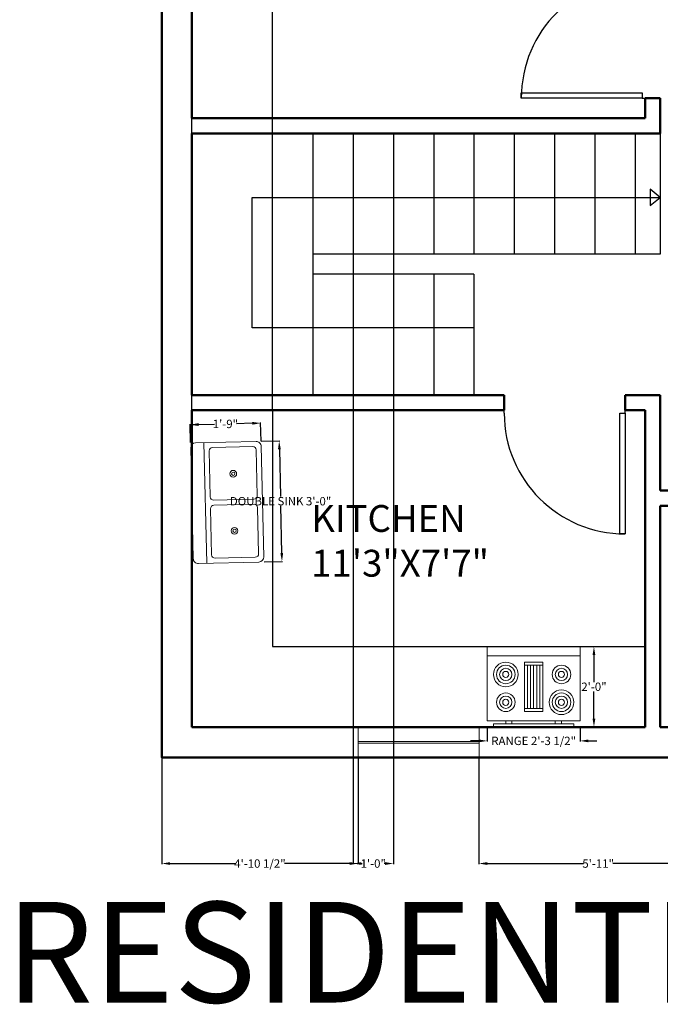
# Model space of a CAD drawing. Units: inches. Extents: x 14 to 510, y 5 to 635.
# Tile 1 of 3: x 14 to 205, y 5 to 299. Entities that reach past the tile are written whole.
import ezdxf

# ---------------------------------------------------------------- set-up
doc = ezdxf.new("R2010")
doc.units = ezdxf.units.IN
doc.header["$MEASUREMENT"] = 0
for name, color, linetype, lineweight in [('A-ANNO-DIMS', 210, 'Continuous', 18), ('A-AREA-IDEN', 210, 'Continuous', 25), ('A-FLOR-CASE', 100, 'Continuous', 25), ('A-FLOR-FIXT', 100, 'Continuous', 18), ('DOOR', 20, 'Continuous', 25), ('EQUIPMENT', 100, 'Continuous', 18), ('STAIRCASE', 50, 'Continuous', 25), ('TEXT', 210, 'Continuous', 35), ('WALL', 40, 'Continuous', 50), ('WINDOW', 131, 'Continuous', 18)]:
    doc.layers.add(name, color=color, linetype=linetype, lineweight=lineweight)
doc.styles.get("Standard").update_dxf_attribs({"font": 'arial.ttf'})
doc.dimstyles.get("Standard").update_dxf_attribs({"dimtxt": 2.5, "dimasz": 2.5, "dimexe": 0.18, "dimexo": 0.0625, "dimgap": 0.09, "dimtad": 0, "dimtih": 1, "dimtoh": 1, "dimzin": 0, "dimdsep": 46, "dimlunit": 3, "dimtxsty": 'Standard', "dimcen": 0.09, "dimadec": 0, "dimazin": 0, "dimtfac": 1, "dimtofl": 0, "dimtmove": 0, "dimatfit": 3, "dimfxl": 1, "dimtolj": 1, "dimtzin": 0, "dimarcsym": 0})

# ---------------------------------------------------------------- blocks, each defined once
blk = doc.blocks.new('*U2')
for p, q in [((0, 0), (0, -6)), ((40, 0), (40, -6))]:
    blk.add_line(p, q)
blk.add_lwpolyline([(0, 0), (0, 40), (1.75, 40), (1.75, 0)], close=True)
blk.add_arc((0, 0), 40, 0, 90)
blk = doc.blocks.new('Range-Oven - 30 in top')
for p, q in [((0, -3), (30, -3)), ((12, -6), (18, -6)), ((13, -20), (13, -6)), ((14, -6), (14, -20)), ((15, -20), (15, -6)), ((16, -6), (16, -20)), ((17, -20), (17, -6)), ((18, -20), (12, -20)), ((6, -24), (6, -25)), ((8, -25), (8, -24)), ((22, -25), (22, -24)), ((24, -24), (24, -25))]:
    blk.add_line(p, q)
for points in [[(0, -24), (0, 0), (30, 0), (30, -24)], [(12, -21), (12, -5), (18, -5), (18, -21)], [(2, -26), (2, -25), (28, -25), (28, -26)]]:
    blk.add_lwpolyline(points, close=True)
for centre, radius in [((6, -9), 4), ((6, -9), 3), ((24, -9), 3), ((6, -9), 2), ((6, -9), 1), ((24, -9), 2), ((24, -9), 1), ((6, -18), 3), ((24, -18), 4), ((24, -18), 3), ((6, -18), 2), ((6, -18), 1), ((24, -18), 2), ((24, -18), 1)]:
    blk.add_circle(centre, radius)
blk = doc.blocks.new('Sink-double - 36 in top')
for p, q in [((-18, -4), (18, -4)), ((-0.75, -18.5), (-0.75, -6.5)), ((0.75, -6.5), (0.75, -18.5))]:
    blk.add_line(p, q)
for points in [[(-16.5, 0), (16.5, 0)], [(-18, -19.5), (-18, -1.5)], [(18, -1.5), (18, -19.5)], [(-15.5, -5.5), (-1.75, -5.5)], [(1.75, -5.5), (15.5, -5.5)], [(-16.5, -18.5), (-16.5, -6.5)], [(16.5, -6.5), (16.5, -18.5)], [(-1.75, -19.5), (-15.5, -19.5)], [(15.5, -19.5), (1.75, -19.5)], [(16.5, -21), (-16.5, -21)]]:
    blk.add_lwpolyline(points)
for centre, radius in [((-8.5, -12.5), 1), ((8.5, -12.5), 1), ((-8.5, -12.5), 0.5), ((8.5, -12.5), 0.5)]:
    blk.add_circle(centre, radius)
for centre, radius, start, end in [((-16.5, -1.5), 1.5, 90, 180), ((16.5, -1.5), 1.5, 0, 90), ((-15.5, -6.5), 1, 90, 180), ((-1.75, -6.5), 1, 0, 90), ((1.75, -6.5), 1, 90, 180), ((15.5, -6.5), 1, 0, 90), ((-16.5, -19.5), 1.5, 180, 270), ((-15.5, -18.5), 1, 180, 270), ((-1.75, -18.5), 1, 270, 0), ((1.75, -18.5), 1, 180, 270), ((15.5, -18.5), 1, 270, 0), ((16.5, -19.5), 1.5, 270, 0)]:
    blk.add_arc(centre, radius, start, end)
blk = doc.blocks.new('WIN-36IN')
for p, q in [((0, 4.75), (36, 4.75)), ((0, 4.25), (36, 4.25))]:
    blk.add_line(p, q)
blk.add_lwpolyline([(0, 0), (36, 0), (36, 9), (0, 9)], close=True)
blk = doc.blocks.new('*D35')
at = {"layer": 'A-ANNO-DIMS', "color": 0, "lineweight": -2, "transparency": 16777216}
for p, q in [((153.57, 88.05), (153.57, 83.79)), ((181.2, 88.05), (181.2, 83.79)), ((151.07, 83.97), (148.57, 83.97)), ((183.7, 83.97), (186.2, 83.97))]:
    blk.add_line(p, q, dxfattribs=at)
at = {"layer": 'A-ANNO-DIMS', "color": 0, "transparency": 16777216}
for points in [[(151.07, 84.38), (151.07, 83.55), (153.57, 83.97)], [(183.7, 84.38), (183.7, 83.55), (181.2, 83.97)]]:
    blk.add_solid(points, dxfattribs=at)
at = {"layer": 'Defpoints', "color": 0, "transparency": 16777216}
for p in [(153.57, 88.11), (181.2, 88.11), (181.2, 83.97)]:
    blk.add_point(p, dxfattribs=at)
at = {"layer": 'A-ANNO-DIMS', "color": 0, "transparency": 16777216, "insert": (167.39, 83.97), "char_height": 2.5, "attachment_point": 5}
blk.add_mtext('\\A1;RANGE 2\'-3 1/2"', dxfattribs=at)
blk = doc.blocks.new('*D36')
at = {"layer": 'A-ANNO-DIMS', "color": 0, "lineweight": -2, "transparency": 16777216}
for p, q in [((181.27, 112.06), (185.53, 112.06)), ((185.35, 109.56), (185.35, 101.45)), ((185.35, 90.61), (185.35, 98.72)), ((181.27, 88.11), (185.53, 88.11))]:
    blk.add_line(p, q, dxfattribs=at)
at = {"layer": 'A-ANNO-DIMS', "color": 0, "transparency": 16777216}
for points in [[(184.93, 109.56), (185.76, 109.56), (185.35, 112.06)], [(184.93, 90.61), (185.76, 90.61), (185.35, 88.11)]]:
    blk.add_solid(points, dxfattribs=at)
at = {"layer": 'Defpoints', "color": 0, "transparency": 16777216}
for p in [(181.2, 112.06), (185.35, 112.06), (181.2, 88.11)]:
    blk.add_point(p, dxfattribs=at)
at = {"layer": 'A-ANNO-DIMS', "color": 0, "transparency": 16777216, "insert": (185.35, 100.09), "char_height": 2.5, "attachment_point": 5}
blk.add_mtext('\\A1;2\'-0"', dxfattribs=at)
blk = doc.blocks.new('*D37')
at = {"layer": 'A-ANNO-DIMS', "color": 0, "lineweight": -2, "transparency": 16777216}
for p, q in [((86.26, 173.29), (91.77, 173.41)), ((91.65, 170.91), (91.97, 156.8)), ((92.36, 139.92), (92.04, 154.03)), ((87.08, 137.3), (92.6, 137.42))]:
    blk.add_line(p, q, dxfattribs=at)
at = {"layer": 'A-ANNO-DIMS', "color": 0, "transparency": 16777216}
for points in [[(92.07, 170.92), (91.23, 170.9), (91.59, 173.41)], [(92.78, 139.93), (91.94, 139.91), (92.42, 137.42)]]:
    blk.add_solid(points, dxfattribs=at)
at = {"layer": 'Defpoints', "color": 0, "transparency": 16777216}
for p in [(86.19, 173.29), (91.59, 173.41), (87.02, 137.29)]:
    blk.add_point(p, dxfattribs=at)
at = {"layer": 'A-ANNO-DIMS', "color": 0, "transparency": 16777216, "insert": (92, 155.41), "char_height": 2.5, "attachment_point": 5}
blk.add_mtext('\\A1;DOUBLE SINK 3\'-0"', dxfattribs=at)
blk = doc.blocks.new('*D38')
at = {"layer": 'A-ANNO-DIMS', "color": 0, "lineweight": -2, "transparency": 16777216}
for p, q in [((65.2, 172.87), (65.07, 178.38)), ((67.57, 178.26), (72.28, 178.37)), ((83.57, 178.63), (78.87, 178.52)), ((86.19, 173.35), (86.06, 178.86))]:
    blk.add_line(p, q, dxfattribs=at)
at = {"layer": 'A-ANNO-DIMS', "color": 0, "transparency": 16777216}
for points in [[(83.56, 179.04), (83.58, 178.21), (86.07, 178.68)], [(67.56, 178.68), (67.58, 177.84), (65.07, 178.2)]]:
    blk.add_solid(points, dxfattribs=at)
at = {"layer": 'Defpoints', "color": 0, "transparency": 16777216}
for p in [(65.07, 178.2), (86.19, 173.29), (65.2, 172.8)]:
    blk.add_point(p, dxfattribs=at)
at = {"layer": 'A-ANNO-DIMS', "color": 0, "transparency": 16777216, "insert": (75.57, 178.44), "char_height": 2.5, "attachment_point": 5}
blk.add_mtext('\\A1;1\'-9"', dxfattribs=at)
blk = doc.blocks.new('*D42')
at = {"layer": 'A-ANNO-DIMS', "color": 0, "lineweight": -2, "transparency": 16777216}
for p, q in [((56.61, 79), (56.61, 47.23)), ((115.11, 79), (115.11, 47.23)), ((59.11, 47.41), (78.51, 47.41)), ((112.61, 47.41), (93.21, 47.41))]:
    blk.add_line(p, q, dxfattribs=at)
at = {"layer": 'A-ANNO-DIMS', "color": 0, "transparency": 16777216}
for points in [[(59.11, 47.83), (59.11, 46.99), (56.61, 47.41)], [(112.61, 47.83), (112.61, 46.99), (115.11, 47.41)]]:
    blk.add_solid(points, dxfattribs=at)
at = {"layer": 'Defpoints', "color": 0, "transparency": 16777216}
for p in [(56.61, 79.06), (115.11, 79.06), (115.11, 47.41)]:
    blk.add_point(p, dxfattribs=at)
at = {"layer": 'A-ANNO-DIMS', "color": 0, "transparency": 16777216, "insert": (85.86, 47.41), "char_height": 2.5, "attachment_point": 5}
blk.add_mtext('\\A1;4\'-10 1/2"', dxfattribs=at)
blk = doc.blocks.new('*D43')
at = {"layer": 'A-ANNO-DIMS', "color": 0, "lineweight": -2, "transparency": 16777216}
for p, q in [((151.11, 79), (151.11, 47.23)), ((222.11, 79), (222.11, 47.23)), ((153.61, 47.41), (182.23, 47.41)), ((219.61, 47.41), (190.99, 47.41))]:
    blk.add_line(p, q, dxfattribs=at)
at = {"layer": 'A-ANNO-DIMS', "color": 0, "transparency": 16777216}
for points in [[(153.61, 47.83), (153.61, 46.99), (151.11, 47.41)], [(219.61, 47.83), (219.61, 46.99), (222.11, 47.41)]]:
    blk.add_solid(points, dxfattribs=at)
at = {"layer": 'Defpoints', "color": 0, "transparency": 16777216}
for p in [(151.11, 79.06), (222.11, 79.06), (222.11, 47.41)]:
    blk.add_point(p, dxfattribs=at)
at = {"layer": 'A-ANNO-DIMS', "color": 0, "transparency": 16777216, "insert": (186.61, 47.41), "char_height": 2.5, "attachment_point": 5}
blk.add_mtext('\\A1;5\'-11"', dxfattribs=at)
blk = doc.blocks.new('*D51')
at = {"layer": 'A-ANNO-DIMS', "color": 0, "lineweight": -2, "transparency": 16777216}
for p, q in [((113.61, 265), (113.61, 47.23)), ((125.61, 265), (125.61, 47.23)), ((116.11, 47.41), (116.32, 47.41)), ((123.11, 47.41), (122.91, 47.41))]:
    blk.add_line(p, q, dxfattribs=at)
at = {"layer": 'A-ANNO-DIMS', "color": 0, "transparency": 16777216}
for points in [[(116.11, 47.83), (116.11, 46.99), (113.61, 47.41)], [(123.11, 47.83), (123.11, 46.99), (125.61, 47.41)]]:
    blk.add_solid(points, dxfattribs=at)
at = {"layer": 'Defpoints', "color": 0, "transparency": 16777216}
for p in [(113.61, 265.06), (125.61, 265.06), (125.61, 47.41)]:
    blk.add_point(p, dxfattribs=at)
at = {"layer": 'A-ANNO-DIMS', "color": 0, "transparency": 16777216, "insert": (119.61, 47.41), "char_height": 2.5, "attachment_point": 5}
blk.add_mtext('\\A1;1\'-0"', dxfattribs=at)
blk = doc.blocks.new('*D56')
at = {"layer": 'A-ANNO-DIMS', "color": 0, "lineweight": -2, "transparency": 16777216}
for p, q in [((65.61, 182.62), (65.61, 590.89)), ((68.11, 590.71), (74.18, 590.71)), ((87.11, 590.71), (81.05, 590.71)), ((89.61, 182.62), (89.61, 590.89))]:
    blk.add_line(p, q, dxfattribs=at)
at = {"layer": 'A-ANNO-DIMS', "color": 0, "transparency": 16777216}
for points in [[(68.11, 591.13), (68.11, 590.29), (65.61, 590.71)], [(87.11, 591.13), (87.11, 590.29), (89.61, 590.71)]]:
    blk.add_solid(points, dxfattribs=at)
at = {"layer": 'Defpoints', "color": 0, "transparency": 16777216}
for p in [(89.61, 590.71), (65.61, 182.56), (89.61, 182.56)]:
    blk.add_point(p, dxfattribs=at)
at = {"layer": 'A-ANNO-DIMS', "color": 0, "transparency": 16777216, "insert": (77.61, 590.71), "char_height": 2.5, "attachment_point": 5}
blk.add_mtext('\\A1;2\'-0"', dxfattribs=at)

msp = doc.modelspace()

# ---------------------------------------------------------------- linework, layer by layer
at = {"layer": 'A-FLOR-CASE'}
for p, q in [((89.611, 182.561), (89.611, 112.061)), ((89.611, 112.061), (200.611, 112.061))]:
    msp.add_line(p, q, dxfattribs=at)
at = {"layer": 'STAIRCASE'}
for p, q in [((101.611, 265.061), (101.611, 187.061)), ((113.611, 265.061), (113.611, 229.061)), ((125.611, 265.061), (125.611, 229.061)), ((137.611, 265.061), (137.611, 229.061)), ((149.611, 265.061), (149.611, 229.061)), ((161.611, 265.061), (161.611, 229.061)), ((173.611, 265.061), (173.611, 229.061)), ((185.611, 265.061), (185.611, 229.061)), ((197.611, 265.061), (197.611, 229.061)), ((205.111, 265.061), (205.111, 229.061)), ((205.111, 245.906), (202.115, 248.4)), ((202.115, 248.4), (202.115, 243.6)), ((83.587, 207.041), (83.587, 245.906)), ((83.587, 245.906), (205.111, 245.906)), ((202.115, 243.6), (205.111, 245.906)), ((205.111, 229.061), (101.611, 229.061)), ((149.611, 223.061), (101.611, 223.061)), ((113.611, 223.061), (113.611, 187.061)), ((125.611, 223.061), (125.611, 187.061)), ((137.611, 223.061), (137.611, 187.061)), ((149.611, 223.061), (149.611, 187.061)), ((149.611, 207.041), (83.587, 207.041))]:
    msp.add_line(p, q, dxfattribs=at)
at = {"layer": 'WALL'}
for p, q in [((65.611, 550.061), (65.611, 269.561)), ((200.611, 275.561), (205.111, 275.561)), ((200.611, 275.561), (200.611, 269.561)), ((205.111, 275.561), (205.111, 265.061)), ((200.611, 269.561), (65.611, 269.561)), ((205.111, 265.061), (65.611, 265.061)), ((65.611, 265.061), (65.611, 187.061)), ((158.611, 187.061), (65.611, 187.061)), ((158.611, 182.561), (158.611, 187.061)), ((205.111, 187.061), (194.611, 187.061)), ((194.611, 182.561), (194.611, 187.061)), ((205.111, 187.061), (205.111, 182.561)), ((65.611, 182.561), (65.611, 88.061)), ((158.611, 182.561), (65.611, 182.561)), ((200.611, 182.561), (194.611, 182.561)), ((200.611, 182.561), (200.611, 88.061)), ((205.111, 182.561), (205.111, 158.561)), ((205.111, 158.561), (211.111, 158.561)), ((205.111, 154.061), (211.111, 154.061)), ((205.111, 154.061), (205.111, 88.061)), ((65.611, 88.061), (200.611, 88.061)), ((205.111, 88.061), (275.111, 88.061))]:
    msp.add_line(p, q, dxfattribs=at)
msp.add_lwpolyline([(331.111, 79.061), (416.611, 79.061), (416.611, 559.061), (56.611, 559.061), (56.611, 79.061), (279.611, 79.061)], dxfattribs=at)

# ---------------------------------------------------------------- block references
at = {"layer": 'A-FLOR-FIXT', "rotation": 91.3142792791285}
msp.add_blockref('Sink-double - 36 in top', (65.611, 154.808), dxfattribs=at)
at = {"layer": 'DOOR'}
for p, xscale, yscale, zscale, rotation in [((199.711, 275.561), 0.9, 0.9, 0.9, 90), ((194.611, 181.661), 0.8999999999999992, 0.8999999999999992, 0.8999999999999992, 180)]:
    msp.add_blockref('*U2', p, dxfattribs=dict(at, xscale=xscale, yscale=yscale, zscale=zscale, rotation=rotation))
at = {"layer": 'EQUIPMENT', "xscale": 0.9211102661868, "yscale": 0.9211102661868, "zscale": 0.9211102661868}
msp.add_blockref('Range-Oven - 30 in top', (153.57, 112.061), dxfattribs=at)
at = {"layer": 'WINDOW'}
msp.add_blockref('WIN-36IN', (115.111, 79.061), dxfattribs=at)

# ---------------------------------------------------------------- texts
at = {"layer": 'A-AREA-IDEN', "insert": (101.12, 154.264), "char_height": 8, "attachment_point": 1}
msp.add_mtext_dynamic_manual_height_columns('KITCHEN\\P11\'3"X7\'7"', width=74.81964, gutter_width=1, heights=[0], dxfattribs=at)
at = {"layer": 'TEXT', "insert": (10.17, 35.979), "char_height": 30, "attachment_point": 1}
msp.add_mtext_dynamic_manual_height_columns('RESIDENTIAL FLOOR PLAN', width=650.16695, gutter_width=1, heights=[0], dxfattribs=at)

# ---------------------------------------------------------------- dimensions: what is measured, and where the dimension line sits
at = {"layer": 'A-ANNO-DIMS'}
for base, p1, p2, picture, middle in [((89.611, 590.711), (65.611, 182.561), (89.611, 182.561), '*D56', (77.611, 590.711)), ((125.611, 47.411), (113.611, 265.061), (125.611, 265.061), '*D51', (119.611, 47.411)), ((115.111, 47.411), (56.611, 79.061), (115.111, 79.061), '*D42', (85.861, 47.411)), ((222.111, 47.411), (151.111, 79.061), (222.111, 79.061), '*D43', (186.611, 47.411))]:
    dim = msp.add_linear_dim(base=base, p1=p1, p2=p2, dimstyle='Standard', override={"dimdec": 1, "dimlfac": 1, "dimrnd": 0, "dimzin": 1, "dimdsep": 46, "dimlunit": 4, "dimfrac": 2}, dxfattribs=at)
    dim.commit()
    dim.dimension.update_dxf_attribs({"geometry": picture, "text_midpoint": middle})
for base, p1, p2, angle, picture, middle in [((65.074, 178.202), (86.193, 173.285), (65.198, 172.804), 181.31428, '*D38', (75.572, 178.443)), ((185.348, 112.061), (181.203, 88.112), (181.203, 112.061), 90, '*D36', (185.348, 100.087))]:
    dim = msp.add_linear_dim(base=base, p1=p1, p2=p2, angle=angle, dimstyle='Standard', override={"dimdec": 1, "dimlfac": 1, "dimrnd": 0, "dimzin": 1, "dimdsep": 46, "dimlunit": 4, "dimfrac": 2}, dxfattribs=at)
    dim.commit()
    dim.dimension.update_dxf_attribs({"geometry": picture, "text_midpoint": middle})
dim = msp.add_linear_dim(base=(91.591, 173.409), p1=(87.018, 137.295), p2=(86.193, 173.285), angle=91.31428, text='DOUBLE SINK <>', dimstyle='Standard', override={"dimdec": 1, "dimlfac": 1, "dimrnd": 0, "dimzin": 1, "dimdsep": 46, "dimlunit": 4, "dimfrac": 2}, dxfattribs=at)
dim.commit()
dim.dimension.update_dxf_attribs({"geometry": '*D37', "text_midpoint": (92.004, 155.414)})
dim = msp.add_linear_dim(base=(181.203, 83.967), p1=(153.57, 88.112), p2=(181.203, 88.112), text='RANGE <>', dimstyle='Standard', override={"dimdec": 1, "dimlfac": 1, "dimrnd": 0, "dimzin": 1, "dimdsep": 46, "dimlunit": 4, "dimfrac": 2}, dxfattribs=at)
dim.commit()
dim.dimension.update_dxf_attribs({"geometry": '*D35', "text_midpoint": (167.387, 83.967)})

doc.saveas('drawing.dxf')
